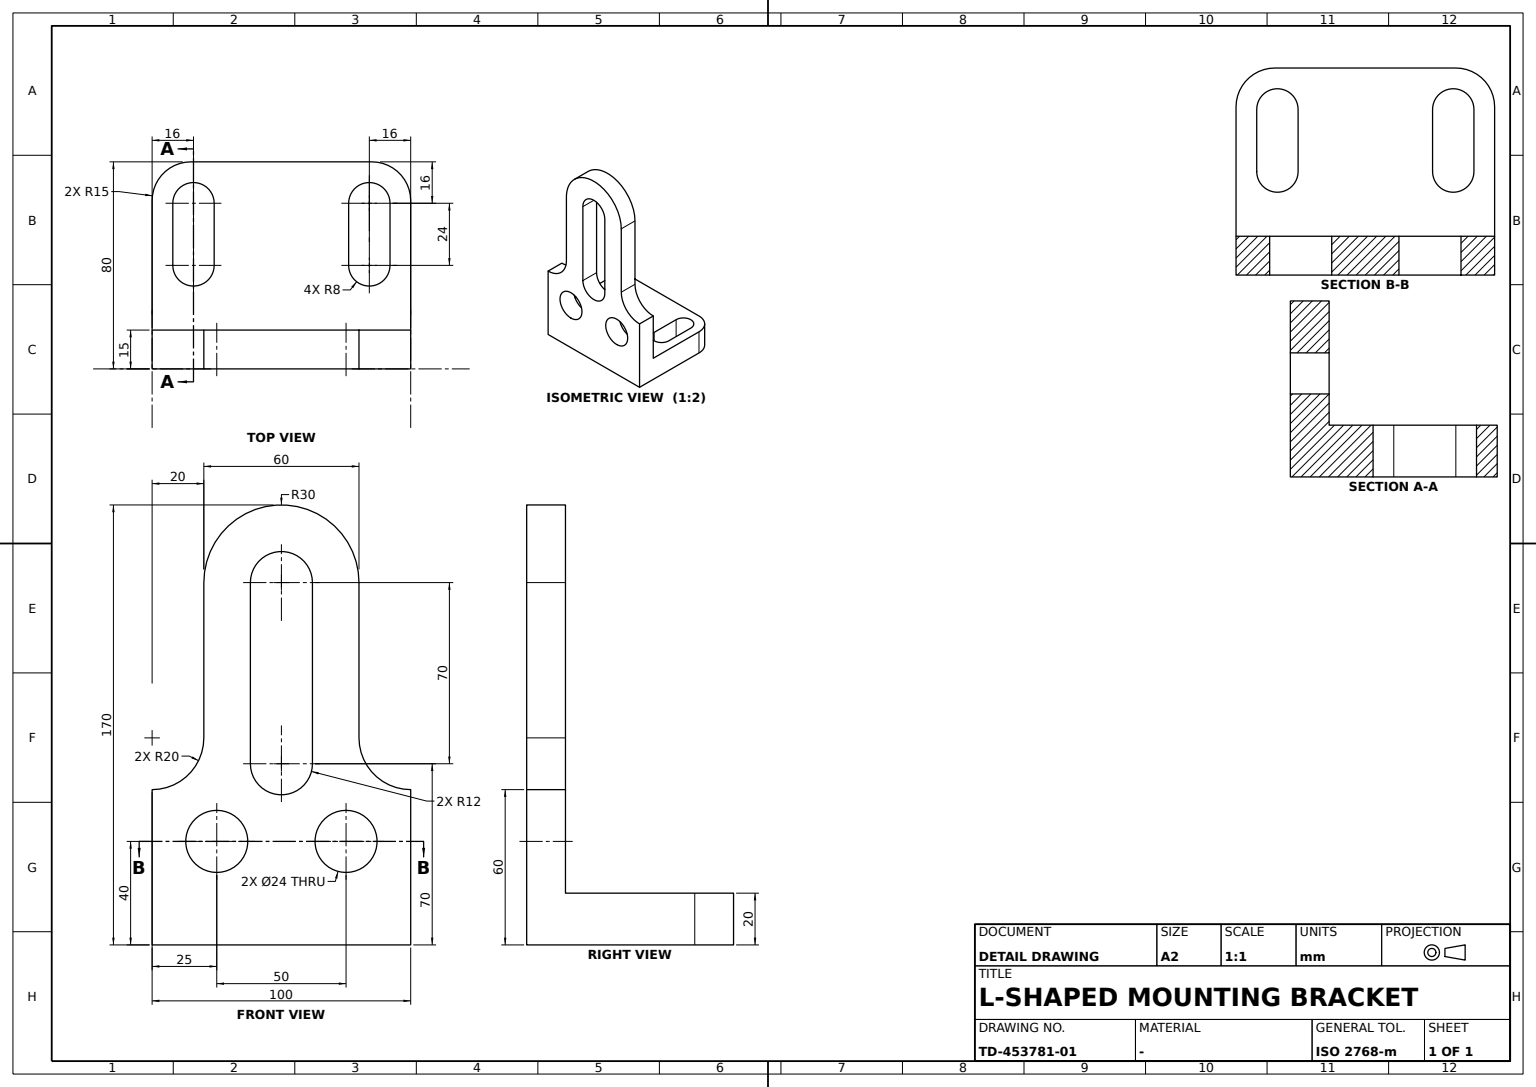
CATIA V5 part; units mm, degrees
sketch "Sketch1" plane through (0, 0, 0) normal (0, 0, 1) x (0, 1, 0)
  point P0 (0, 50)
  line L0 (0, 50) -> (80, 50)
  line L1 (80, 50) -> (80, -50)
  line L2 (80, -50) -> (0, -50)
  line L3 (0, -50) -> (0, 50)
  arc A0 (40, 42) -> (40, 26) centre (40, 34) ccw
  point P1 (40, 34)
  arc A1 (64, 26) -> (64, 42) centre (64, 34) ccw
  point P2 (64, 34)
  point P3 (40, 42)
  line L4 (40, 42) -> (64, 42)
  point P4 (64, 42)
  point P5 (40, 26)
  line L5 (40, 26) -> (64, 26)
  point P6 (64, 26)
  point P7 (64, -26)
  point P8 (40, -26)
  line L6 (40, -26) -> (64, -26)
  point P9 (64, -42)
  point P10 (40, -42)
  line L7 (40, -42) -> (64, -42)
  arc A2 (40, -42) -> (40, -26) centre (40, -34) cw
  arc A3 (64, -26) -> (64, -42) centre (64, -34) cw
  dimension "length L2" = 80
  dimension "length L1" = 100
  dimension "radius A0" = 8
  dimension "distance P1 P2 x axis" = 24
  dimension "distance L4 L0" = 8
  dimension "distance L1 P2" = 16
  constraint coincidence P0 y-axis
  constraint horizontal L0 x-axis
  constraint horizontal L2 x-axis
  constraint horizontal L4 x-axis
  constraint horizontal L5 x-axis
  constraint vertical L1 y-axis
  constraint vertical L3 y-axis
  constraint symmetry L0 L2 x-axis
  constraint symmetry P6 P7 x-axis
  constraint symmetry P5 P8 x-axis
  constraint symmetry L5 L6 x-axis
  constraint symmetry P4 P9 x-axis
  constraint symmetry P3 P10 x-axis
  constraint symmetry L4 L7 x-axis
  constraint symmetry A0 A2 x-axis
  constraint symmetry A1 A3 x-axis
  constraint tangency L4 A1
  constraint tangency L4 A0
  constraint tangency L5 A0
  constraint tangency L5 A1
extrude "Pad1" add sketch "Sketch1" along normal mid plane 20
fillet "Fillet1" radius 15 2 edges at (-50, 80, 0) (50, 80, 0)
sketch "Sketch2" plane through (0, 0, 0) normal (0, -1, 0) x (1, 0, 0)
  point P0 (-50, 10)
  line L0 (-50, 10) -> (-50, 50)
  line L1 (-50, 50) -> (-30, 50)
  line L2 (-30, 50) -> (-30, 130)
  line L3 (30, 130) -> (30, 50)
  point P1 (30, 50)
  line L4 (30, 50) -> (50, 50)
  line L5 (50, 50) -> (50, 10)
  point P2 (50, 10)
  point P3 (50, 10)
  point P4 (-50, 10)
  arc A0 (30, 130) -> (-30, 130) centre (0, 130) ccw
  point P5 (0, 130)
  circle A1 centre (-25, 30) radius 12
  point P6 (-25, 30)
  circle A2 centre (25, 30) radius 12
  point P7 (25, 30)
  arc A3 (12, 130) -> (-12, 130) centre (0, 130) ccw
  arc A4 (-12, 60) -> (12, 60) centre (0, 60) ccw
  point P8 (0, 60)
  point P9 (-12, 130)
  line L6 (-12, 130) -> (-12, 60)
  point P10 (-12, 60)
  point P11 (12, 60)
  point P12 (12, 130)
  line L7 (12, 130) -> (12, 60)
  point P13 (-12, 60)
  point P14 (12, 60)
  line L8 (-50, 10) -> (50, 10) construction
  line L9 (-50, 10) -> (50, 10)
  point P15 (-50, 10)
  point P16 (50, 10)
  dimension "length L1" = 20
  dimension "length L5" = 40
  dimension "radius A4" = 12
  dimension "distance P5 P8" = 70
  dimension "radius A1" = 12
  dimension "radius A2" = 12
  dimension "distance P6 P7" = 50
  dimension "distance P6 L8" = 20
  dimension "distance x axis P8" = 60
  constraint vertical L0 y-axis
  constraint vertical L2 y-axis
  constraint vertical L3 y-axis
  constraint vertical L5 y-axis
  constraint vertical L6 y-axis
  constraint horizontal L1 x-axis
  constraint horizontal L4 x-axis
  constraint coincidence P1 L1
  constraint coincidence P2 P3
  constraint coincidence P0 P4
  constraint coincidence P8 y-axis
  constraint coincidence P10 A4
  constraint coincidence L7 P14
  constraint coincidence L6 P13
  constraint coincidence P0 P15
  constraint coincidence P2 P16
  constraint coincidence P10 P13
  constraint coincidence P11 P14
  constraint tangency L2 A0
  constraint tangency L3 A0
  constraint tangency L6 A4
  constraint tangency L6 A3
  constraint tangency L7 A3
  constraint symmetry P10 P11 y-axis
  constraint symmetry P9 P12 y-axis
  constraint symmetry L6 L7 y-axis
  constraint symmetry P6 P7 y-axis
extrude "Pad2" add sketch "Sketch2" against normal blind 15
fillet "Fillet2" radius 20 1 edges at (30, 7.5, 50)
mirror "Mirror1" about plane through (0, 0, 0) normal (1, 0, 0)
